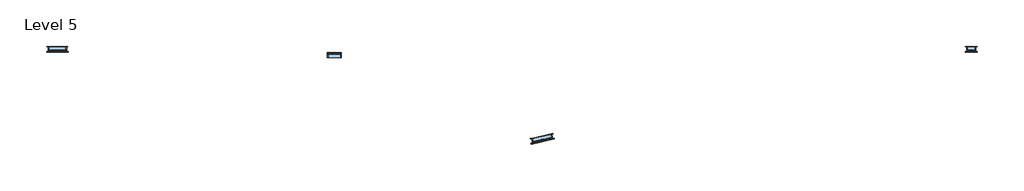
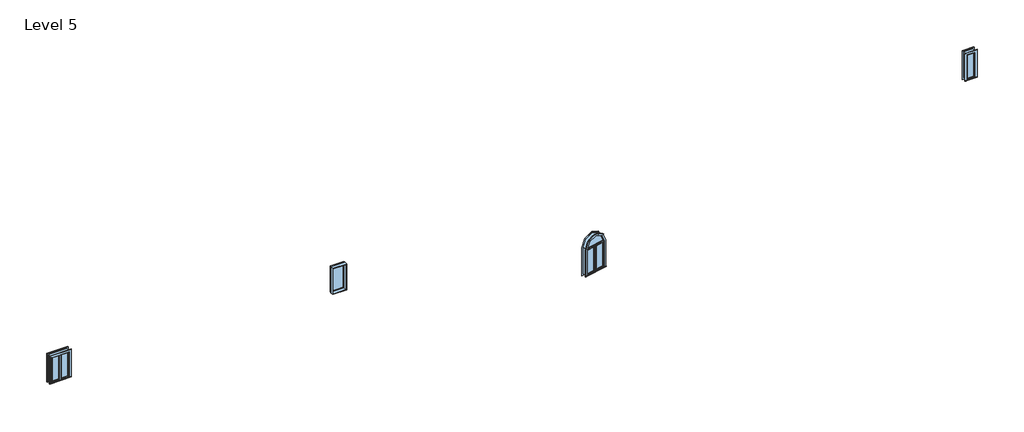
# One storey: 4 windows.
"""IFC4 building model written with IfcOpenShell, lengths in millimetres."""

from ifc_helpers import new_model, si_unit, origin, place, context, project, spatial, transform, mapped, element, save
from components import window_cf4adaea, window_a765b88f, window_bb17773d, window_80bd9af0

model = new_model("IFC4")

# Units and contexts
model_context = context("Model", 3, world=origin())
ifc_project = project(units=[si_unit("LENGTHUNIT", "METRE", prefix="MILLI")], contexts=[model_context])

# Site, building, storey
site = spatial("IfcSite", under=ifc_project)
building = spatial("IfcBuilding", under=site)
storey = spatial("IfcBuildingStorey", under=building, Name="Level 5", Elevation=9448.8)

# Windows
placement = place(None, origin())
window_shape = window_cf4adaea(model_context)
element("IfcWindow", 1, ObjectType="36\" x 48\"", at=placement, inside=storey, context=model_context, shape_type="MappedRepresentation", body=[
    mapped(window_shape, transform((2543.0469577, -16304.4969358, 9448.8), x_axis=(-0.9753253237109197, -0.2207725366257989, 0.0), y_axis=(0.2207725366257989, -0.9753253237109197, 0.0), z_axis=(0.0, 0.0, 1.0))),
])
window_2_shape = window_a765b88f(model_context)
element("IfcWindow", 2, ObjectType="Awning with Trim : 16\" x 48\"", at=placement, inside=storey, context=model_context, shape_type="MappedRepresentation", body=[
    mapped(window_2_shape, transform((21425.814721, -12354.7237084, 9448.8), x_axis=(-1.0, 0.0, 0.0), y_axis=(0.0, -1.0, 0.0), z_axis=(0.0, 0.0, 1.0))),
])
window_3_shape = window_bb17773d(model_context)
element("IfcWindow", 3, ObjectType="Casement Dbl with Trim : 32\" x 48\"", at=placement, inside=storey, context=model_context, shape_type="MappedRepresentation", body=[
    mapped(window_3_shape, transform((-18807.785279, -12335.6737084, 9448.8), x_axis=(-1.0, 0.0, 0.0), y_axis=(0.0, -1.0, 0.0), z_axis=(0.0, 0.0, 1.0))),
])
window_4_shape = window_80bd9af0(model_context)
element("IfcWindow", 4, ObjectType="Fixed : 24\" x 48\"", at=placement, inside=storey, context=model_context, shape_type="MappedRepresentation", body=[
    mapped(window_4_shape, transform((-6577.685279, -12617.2007309, 9448.8), x_axis=(1.0, 0.0, 0.0), y_axis=(0.0, 1.0, 0.0), z_axis=(0.0, 0.0, 1.0))),
])

save(model, "model.ifc")

# Revit data of these elements
# Type "36\" x 48\""
#   Type Mark = "38"
#   Construction Type Id = "SGL"
#   Assembly Code = "B2020100"
#   Analytic Construction = "Large single-glazed windows"
#   Visual Light Transmittance = 0.9
#   Solar Heat Gain Coefficient = 0.86
#   Heat Transfer Coefficient (U) = 0.979472 BTU/(h·ft²·°F)
#   Height = 4' - 0"
#   Default Sill Height = 3' - 0"
#   Trim Projection - Ext. = 0' - 0 1/2"
#   Trim Projection - Int. = 0' - 0 3/4"
#   Trim Width - Exterior = 0' - 3 1/2"
#   Trim Width - Interior = 0' - 3 1/2"
#   Width = 3' - 0"
#   Window Inset = 0' - 0 3/4"
#   Define Thermal Properties by = 1
#   Glass Pane Material = Glass
#   Sash Material = Sash
#   Trim Exterior Material = Trim
#   Trim Interior Material = Trim
#   Wall Closure = (empty or 0)
# Type "Awning with Trim : 16\" x 48\""
#   Type Mark = "14"
#   Construction Type Id = "GSP4R"
#   Assembly Code = "B2020100"
#   Analytic Construction = "1/8 in Pilkington single glazing"
#   Visual Light Transmittance = 0.9
#   Solar Heat Gain Coefficient = 0.78
#   Heat Transfer Coefficient (U) = 0.6496 BTU/(h·ft²·°F)
#   Height = 4' - 0"
#   Default Sill Height = 3' - 0"
#   Trim Projection - Ext. = 0' - 0 1/2"
#   Trim Projection - Int. = 0' - 0 3/4"
#   Trim Width - Exterior = 0' - 3 1/2"
#   Trim Width - Interior = 0' - 3 1/2"
#   Width = 1' - 4"
#   Window Inset = 0' - 0 3/4"
#   Define Thermal Properties by = 1
#   Glass Pane Material = Glass
#   Sash Material = Sash
#   Trim Exterior Material = Trim
#   Trim Interior Material = Trim
#   Wall Closure = (empty or 0)
# Type "Casement Dbl with Trim : 32\" x 48\""
#   Type Mark = "36"
#   Construction Type Id = "GSP4R"
#   Assembly Code = "B2020100"
#   Analytic Construction = "1/8 in Pilkington single glazing"
#   Visual Light Transmittance = 0.9
#   Solar Heat Gain Coefficient = 0.78
#   Heat Transfer Coefficient (U) = 0.6496 BTU/(h·ft²·°F)
#   Height = 4' - 0"
#   Default Sill Height = 3' - 0"
#   Trim Projection - Ext. = 0' - 0 1/2"
#   Trim Projection - Int. = 0' - 0 3/4"
#   Trim Width - Exterior = 0' - 3 1/2"
#   Trim Width - Interior = 0' - 3 1/2"
#   Width = 2' - 8"
#   Window Inset = 0' - 0 3/4"
#   Define Thermal Properties by = 1
#   Glass Pane Material = Glass
#   Sash Material = Sash
#   Trim Exterior Material = Trim
#   Trim Interior Material = Trim
#   Wall Closure = (empty or 0)
# Type "Fixed : 24\" x 48\""
#   Type Mark = "2"
#   Construction Type Id = "GSP4R"
#   Assembly Code = "B2020100"
#   Analytic Construction = "1/8 in Pilkington single glazing"
#   Visual Light Transmittance = 0.9
#   Solar Heat Gain Coefficient = 0.78
#   Heat Transfer Coefficient (U) = 0.6496 BTU/(h·ft²·°F)
#   Height = 4' - 0"
#   Default Sill Height = 3' - 0"
#   Width = 2' - 0"
#   Window Inset = 0' - 0 3/4"
#   Define Thermal Properties by = 1
#   Glass Pane Material = Glass
#   Sash Material = Sash
#   Wall Closure = (empty or 0)
# Element 1 (IfcWindow, "36\" x 48\"")
#   Mark = "31"
#   Phase Created = New Construction
#   Materials on its faces: "Sash", "Trim", "Glass"
# Element 2 (IfcWindow, "Awning with Trim : 16\" x 48\"")
#   Mark = "65"
#   Phase Created = New Construction
#   Materials on its faces: "Sash", "Trim", "Glass"
# Element 3 (IfcWindow, "Casement Dbl with Trim : 32\" x 48\"")
#   Mark = "48"
#   Phase Created = New Construction
#   Materials on its faces: "Sash", "Trim", "Glass"
# Element 4 (IfcWindow, "Fixed : 24\" x 48\"")
#   Mark = "82"
#   Phase Created = New Construction
#   Materials on its faces: "Sash", "Glass"
# Materials
#   "Glass": class "Glass", colour RGB 0 128 192, transparency 0.75, Description = "Soda Lime Glass", Cost = 0
#   "Sash": class "Wood", colour RGB 224 178 126, transparency 0
#   "Trim": class "Wood", colour RGB 224 178 126, transparency 0
